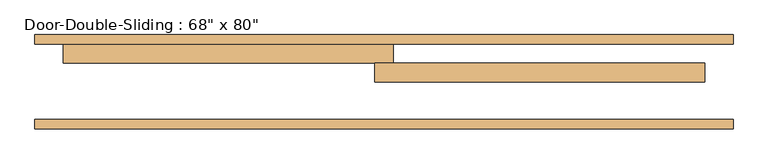
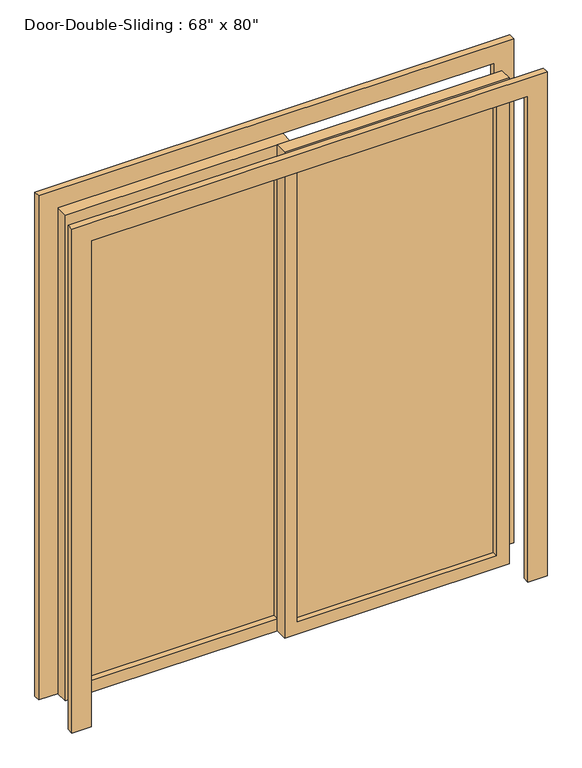
"""IFC4 building model written with IfcOpenShell, lengths in millimetres: door geometry."""

from ifc_helpers import new_model, si_unit, frame, origin, place, context, project, spatial, polyline, outline, extrude, source, transform, mapped, element, save


def door_076b30e0(model_context):
    return source(origin(), model_context, "Body", "SweptSolid", [
        extrude(outline(polyline([(0.0, -939.8), (0.0, -863.6), (2032.0, -863.6), (2032.0, 863.6), (0.0, 863.6), (0.0, 939.8), (2108.2, 939.8), (2108.2, -939.8), (0.0, -939.8)])), frame((0.0, 0.0, 0.0), z_axis=(0.0, 1.0, 0.0), x_axis=(0.0, 0.0, 1.0)), (0.0, 0.0, 1.0), 25.4),
        extrude(outline(polyline([(0.0, 939.8), (2108.2, 939.8), (2108.2, -939.8), (0.0, -939.8), (0.0, -863.6), (2032.0, -863.6), (2032.0, 863.6), (0.0, 863.6), (0.0, 939.8)])), frame((0.0, 228.6, 0.0), z_axis=(0.0, 1.0, 0.0), x_axis=(0.0, 0.0, 1.0)), (0.0, 0.0, 1.0), 25.4),
        extrude(outline(polyline([(2032.0, -25.4), (0.0, -25.4), (0.0, 863.6), (2032.0, 863.6), (2032.0, -25.4)]), holes=[polyline([(1981.2, 25.4), (1981.2, 812.8), (50.8, 812.8), (50.8, 25.4), (1981.2, 25.4)])]), frame((0.0, 127.0, 0.0), z_axis=(0.0, 1.0, 0.0), x_axis=(0.0, 0.0, 1.0)), (0.0, 0.0, 1.0), 50.8),
        extrude(outline(polyline([(2032.0, 25.4), (2032.0, -863.6), (0.0, -863.6), (0.0, 25.4), (2032.0, 25.4)]), holes=[polyline([(1981.2, -25.4), (50.8, -25.4), (50.8, -812.8), (1981.2, -812.8), (1981.2, -25.4)])]), frame((0.0, 177.8, 0.0), z_axis=(0.0, 1.0, 0.0), x_axis=(0.0, 0.0, 1.0)), (0.0, 0.0, 1.0), 50.8),
        extrude(outline(polyline([(25.4, 155.575), (812.8, 155.575), (812.8, 149.225), (25.4, 149.225), (25.4, 155.575)])), frame((0.0, 0.0, 50.8), z_axis=(0.0, 0.0, 1.0), x_axis=(1.0, 0.0, 0.0)), (0.0, 0.0, 1.0), 1930.4),
        extrude(outline(polyline([(-25.4, 200.025), (-812.8, 200.025), (-812.8, 206.375), (-25.4, 206.375), (-25.4, 200.025)])), frame((0.0, 0.0, 50.8), z_axis=(0.0, 0.0, 1.0), x_axis=(1.0, 0.0, 0.0)), (0.0, 0.0, 1.0), 1930.4),
    ])


if __name__ == "__main__":
    model = new_model("IFC4")
    model_context = context("Model", 3, world=origin())
    ifc_project = project(units=[si_unit("LENGTHUNIT", "METRE", prefix="MILLI")], contexts=[model_context])
    site = spatial("IfcSite", under=ifc_project)
    building = spatial("IfcBuilding", under=site)
    placement = place(None, origin())
    door_shape = door_076b30e0(model_context)
    element("IfcDoor", 1, ObjectType="Door-Double-Sliding : 68\" x 80\"", at=placement, inside=building, context=model_context, shape_type="MappedRepresentation", body=[
        mapped(door_shape, transform((0.0, 0.0, 0.0), x_axis=(1.0, 0.0, 0.0), y_axis=(0.0, 1.0, 0.0), z_axis=(0.0, 0.0, 1.0))),
    ])
    save(model, "model.ifc")

# Revit data of these elements
# Type "Door-Double-Sliding : 68\" x 80\""
#   Type Mark = "8"
#   Construction Type Id = "opn-d45"
#   Assembly Code = "C1020"
#   Analytic Construction = "Wood frame, double glass door "
#   Thickness = 0' - 2"
#   Thermal Resistance (R) = 1.8150 (h·ft²·°F)/BTU
#   Heat Transfer Coefficient (U) = 0.5510 BTU/(h·ft²·°F)
#   Height = 6' - 8"
#   Rail Width = 0' - 2"
#   Stiles = 0' - 2"
#   Trim Projection Ext = 0' - 1"
#   Trim Projection Int = 0' - 1"
#   Trim Width = 0' - 3"
#   Width = 5' - 8"
#   Define Thermal Properties by = 1
#   Glazing = Glass
#   Panel Material = Wood - Birch - Solid Stained Light Low Gloss
#   Trim Material = Paint - Sienna
#   Visual Light Transmittance = 0
#   Solar Heat Gain Coefficient = 0
#   Function = (empty or 0)
#   Wall Closure = (empty or 0)
# Element 1 (IfcDoor, "Door-Double-Sliding : 68\" x 80\"")
#   Materials on its faces: "Paint - Sienna", "Wood - Birch - Solid Stained Light Low Gloss", "Glass"
# Materials
#   "Glass": class "Glass", colour RGB 0 128 192, transparency 0.75, Description = "Soda Lime Glass", Cost = 0
#   "Wood - Birch - Solid Stained Light Low Gloss": class "Wood", colour RGB 210 159 95, transparency 0, Cost = 0
#   "Paint - Sienna": colour RGB 118 70 51, transparency 0, Cost = 0
